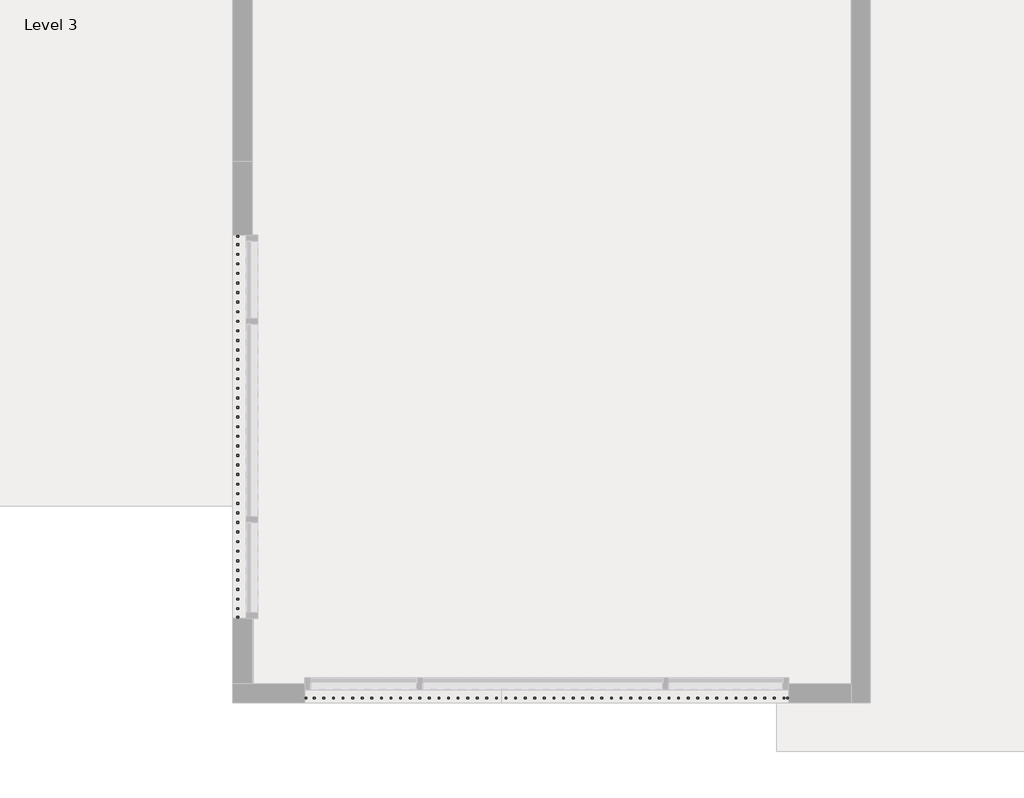
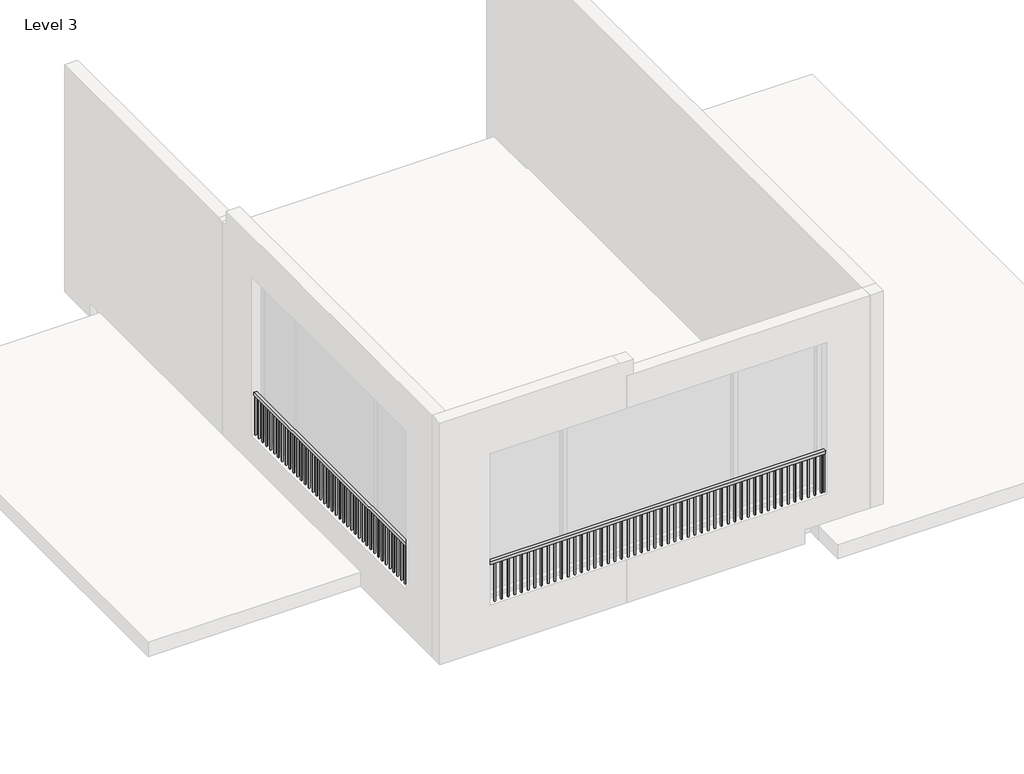
# One storey, part 2 of 2: 2 railings.
"""IFC4 building model written with IfcOpenShell, lengths in millimetres."""

from ifc_helpers import new_model, si_unit, frame, origin, place, context, project, spatial, polyline, outline, extrude, element, save

model = new_model("IFC4")

# Units and contexts
model_context = context("Model", 3, world=origin())
ifc_project = project(units=[si_unit("LENGTHUNIT", "METRE", prefix="MILLI")], contexts=[model_context])

# Site, building, storey
site = spatial("IfcSite", under=ifc_project)
building = spatial("IfcBuilding", under=site)
storey = spatial("IfcBuildingStorey", under=building, Name="Level 3", Elevation=7315.2)

# Railings
placement = place(None, origin())
element("IfcRailing", 1, ObjectType="Handrail - Rectangular", at=placement, inside=storey, context=model_context, shape_type="SweptSolid", body=[
    extrude(outline(polyline([(-11871.2372956, -2267.3372168), (-11871.2372956, -2216.5372168), (-6740.4372956, -2216.5372168), (-6740.4372956, -2267.3372168), (-11871.2372956, -2267.3372168)])), frame((0.0, 0.0, 8636.0), z_axis=(0.0, 0.0, 1.0), x_axis=(1.0, 0.0, 0.0)), (0.0, 0.0, 1.0), 50.8),
    extrude(outline(polyline([(-6800.7622956, -2251.4622168), (-6800.7622956, -2232.4122168), (-6781.7122956, -2232.4122168), (-6781.7122956, -2251.4622168), (-6800.7622956, -2251.4622168)])), frame((0.0, 0.0, 7772.4), z_axis=(0.0, 0.0, 1.0), x_axis=(1.0, 0.0, 0.0)), (0.0, 0.0, 1.0), 863.6),
    extrude(outline(polyline([(-6902.3622956, -2251.4622168), (-6902.3622956, -2232.4122168), (-6883.3122956, -2232.4122168), (-6883.3122956, -2251.4622168), (-6902.3622956, -2251.4622168)])), frame((0.0, 0.0, 7772.4), z_axis=(0.0, 0.0, 1.0), x_axis=(1.0, 0.0, 0.0)), (0.0, 0.0, 1.0), 863.6),
    extrude(outline(polyline([(-7003.9622956, -2251.4622168), (-7003.9622956, -2232.4122168), (-6984.9122956, -2232.4122168), (-6984.9122956, -2251.4622168), (-7003.9622956, -2251.4622168)])), frame((0.0, 0.0, 7772.4), z_axis=(0.0, 0.0, 1.0), x_axis=(1.0, 0.0, 0.0)), (0.0, 0.0, 1.0), 863.6),
    extrude(outline(polyline([(-7105.5622956, -2251.4622168), (-7105.5622956, -2232.4122168), (-7086.5122956, -2232.4122168), (-7086.5122956, -2251.4622168), (-7105.5622956, -2251.4622168)])), frame((0.0, 0.0, 7772.4), z_axis=(0.0, 0.0, 1.0), x_axis=(1.0, 0.0, 0.0)), (0.0, 0.0, 1.0), 863.6),
    extrude(outline(polyline([(-7207.1622956, -2251.4622168), (-7207.1622956, -2232.4122168), (-7188.1122956, -2232.4122168), (-7188.1122956, -2251.4622168), (-7207.1622956, -2251.4622168)])), frame((0.0, 0.0, 7772.4), z_axis=(0.0, 0.0, 1.0), x_axis=(1.0, 0.0, 0.0)), (0.0, 0.0, 1.0), 863.6),
    extrude(outline(polyline([(-7308.7622956, -2251.4622168), (-7308.7622956, -2232.4122168), (-7289.7122956, -2232.4122168), (-7289.7122956, -2251.4622168), (-7308.7622956, -2251.4622168)])), frame((0.0, 0.0, 7772.4), z_axis=(0.0, 0.0, 1.0), x_axis=(1.0, 0.0, 0.0)), (0.0, 0.0, 1.0), 863.6),
    extrude(outline(polyline([(-7410.3622956, -2251.4622168), (-7410.3622956, -2232.4122168), (-7391.3122956, -2232.4122168), (-7391.3122956, -2251.4622168), (-7410.3622956, -2251.4622168)])), frame((0.0, 0.0, 7772.4), z_axis=(0.0, 0.0, 1.0), x_axis=(1.0, 0.0, 0.0)), (0.0, 0.0, 1.0), 863.6),
    extrude(outline(polyline([(-7511.9622956, -2251.4622168), (-7511.9622956, -2232.4122168), (-7492.9122956, -2232.4122168), (-7492.9122956, -2251.4622168), (-7511.9622956, -2251.4622168)])), frame((0.0, 0.0, 7772.4), z_axis=(0.0, 0.0, 1.0), x_axis=(1.0, 0.0, 0.0)), (0.0, 0.0, 1.0), 863.6),
    extrude(outline(polyline([(-7613.5622956, -2251.4622168), (-7613.5622956, -2232.4122168), (-7594.5122956, -2232.4122168), (-7594.5122956, -2251.4622168), (-7613.5622956, -2251.4622168)])), frame((0.0, 0.0, 7772.4), z_axis=(0.0, 0.0, 1.0), x_axis=(1.0, 0.0, 0.0)), (0.0, 0.0, 1.0), 863.6),
    extrude(outline(polyline([(-7715.1622956, -2251.4622168), (-7715.1622956, -2232.4122168), (-7696.1122956, -2232.4122168), (-7696.1122956, -2251.4622168), (-7715.1622956, -2251.4622168)])), frame((0.0, 0.0, 7772.4), z_axis=(0.0, 0.0, 1.0), x_axis=(1.0, 0.0, 0.0)), (0.0, 0.0, 1.0), 863.6),
    extrude(outline(polyline([(-7816.7622956, -2251.4622168), (-7816.7622956, -2232.4122168), (-7797.7122956, -2232.4122168), (-7797.7122956, -2251.4622168), (-7816.7622956, -2251.4622168)])), frame((0.0, 0.0, 7772.4), z_axis=(0.0, 0.0, 1.0), x_axis=(1.0, 0.0, 0.0)), (0.0, 0.0, 1.0), 863.6),
    extrude(outline(polyline([(-7918.3622956, -2251.4622168), (-7918.3622956, -2232.4122168), (-7899.3122956, -2232.4122168), (-7899.3122956, -2251.4622168), (-7918.3622956, -2251.4622168)])), frame((0.0, 0.0, 7772.4), z_axis=(0.0, 0.0, 1.0), x_axis=(1.0, 0.0, 0.0)), (0.0, 0.0, 1.0), 863.6),
    extrude(outline(polyline([(-8019.9622956, -2251.4622168), (-8019.9622956, -2232.4122168), (-8000.9122956, -2232.4122168), (-8000.9122956, -2251.4622168), (-8019.9622956, -2251.4622168)])), frame((0.0, 0.0, 7772.4), z_axis=(0.0, 0.0, 1.0), x_axis=(1.0, 0.0, 0.0)), (0.0, 0.0, 1.0), 863.6),
    extrude(outline(polyline([(-8121.5622956, -2251.4622168), (-8121.5622956, -2232.4122168), (-8102.5122956, -2232.4122168), (-8102.5122956, -2251.4622168), (-8121.5622956, -2251.4622168)])), frame((0.0, 0.0, 7772.4), z_axis=(0.0, 0.0, 1.0), x_axis=(1.0, 0.0, 0.0)), (0.0, 0.0, 1.0), 863.6),
    extrude(outline(polyline([(-8223.1622956, -2251.4622168), (-8223.1622956, -2232.4122168), (-8204.1122956, -2232.4122168), (-8204.1122956, -2251.4622168), (-8223.1622956, -2251.4622168)])), frame((0.0, 0.0, 7772.4), z_axis=(0.0, 0.0, 1.0), x_axis=(1.0, 0.0, 0.0)), (0.0, 0.0, 1.0), 863.6),
    extrude(outline(polyline([(-8324.7622956, -2251.4622168), (-8324.7622956, -2232.4122168), (-8305.7122956, -2232.4122168), (-8305.7122956, -2251.4622168), (-8324.7622956, -2251.4622168)])), frame((0.0, 0.0, 7772.4), z_axis=(0.0, 0.0, 1.0), x_axis=(1.0, 0.0, 0.0)), (0.0, 0.0, 1.0), 863.6),
    extrude(outline(polyline([(-8426.3622956, -2251.4622168), (-8426.3622956, -2232.4122168), (-8407.3122956, -2232.4122168), (-8407.3122956, -2251.4622168), (-8426.3622956, -2251.4622168)])), frame((0.0, 0.0, 7772.4), z_axis=(0.0, 0.0, 1.0), x_axis=(1.0, 0.0, 0.0)), (0.0, 0.0, 1.0), 863.6),
    extrude(outline(polyline([(-8527.9622956, -2251.4622168), (-8527.9622956, -2232.4122168), (-8508.9122956, -2232.4122168), (-8508.9122956, -2251.4622168), (-8527.9622956, -2251.4622168)])), frame((0.0, 0.0, 7772.4), z_axis=(0.0, 0.0, 1.0), x_axis=(1.0, 0.0, 0.0)), (0.0, 0.0, 1.0), 863.6),
    extrude(outline(polyline([(-8629.5622956, -2251.4622168), (-8629.5622956, -2232.4122168), (-8610.5122956, -2232.4122168), (-8610.5122956, -2251.4622168), (-8629.5622956, -2251.4622168)])), frame((0.0, 0.0, 7772.4), z_axis=(0.0, 0.0, 1.0), x_axis=(1.0, 0.0, 0.0)), (0.0, 0.0, 1.0), 863.6),
    extrude(outline(polyline([(-8731.1622956, -2251.4622168), (-8731.1622956, -2232.4122168), (-8712.1122956, -2232.4122168), (-8712.1122956, -2251.4622168), (-8731.1622956, -2251.4622168)])), frame((0.0, 0.0, 7772.4), z_axis=(0.0, 0.0, 1.0), x_axis=(1.0, 0.0, 0.0)), (0.0, 0.0, 1.0), 863.6),
    extrude(outline(polyline([(-8832.7622956, -2251.4622168), (-8832.7622956, -2232.4122168), (-8813.7122956, -2232.4122168), (-8813.7122956, -2251.4622168), (-8832.7622956, -2251.4622168)])), frame((0.0, 0.0, 7772.4), z_axis=(0.0, 0.0, 1.0), x_axis=(1.0, 0.0, 0.0)), (0.0, 0.0, 1.0), 863.6),
    extrude(outline(polyline([(-8934.3622956, -2251.4622168), (-8934.3622956, -2232.4122168), (-8915.3122956, -2232.4122168), (-8915.3122956, -2251.4622168), (-8934.3622956, -2251.4622168)])), frame((0.0, 0.0, 7772.4), z_axis=(0.0, 0.0, 1.0), x_axis=(1.0, 0.0, 0.0)), (0.0, 0.0, 1.0), 863.6),
    extrude(outline(polyline([(-9035.9622956, -2251.4622168), (-9035.9622956, -2232.4122168), (-9016.9122956, -2232.4122168), (-9016.9122956, -2251.4622168), (-9035.9622956, -2251.4622168)])), frame((0.0, 0.0, 7772.4), z_axis=(0.0, 0.0, 1.0), x_axis=(1.0, 0.0, 0.0)), (0.0, 0.0, 1.0), 863.6),
    extrude(outline(polyline([(-9137.5622956, -2251.4622168), (-9137.5622956, -2232.4122168), (-9118.5122956, -2232.4122168), (-9118.5122956, -2251.4622168), (-9137.5622956, -2251.4622168)])), frame((0.0, 0.0, 7772.4), z_axis=(0.0, 0.0, 1.0), x_axis=(1.0, 0.0, 0.0)), (0.0, 0.0, 1.0), 863.6),
    extrude(outline(polyline([(-9239.1622956, -2251.4622168), (-9239.1622956, -2232.4122168), (-9220.1122956, -2232.4122168), (-9220.1122956, -2251.4622168), (-9239.1622956, -2251.4622168)])), frame((0.0, 0.0, 7772.4), z_axis=(0.0, 0.0, 1.0), x_axis=(1.0, 0.0, 0.0)), (0.0, 0.0, 1.0), 863.6),
    extrude(outline(polyline([(-9340.7622956, -2251.4622168), (-9340.7622956, -2232.4122168), (-9321.7122956, -2232.4122168), (-9321.7122956, -2251.4622168), (-9340.7622956, -2251.4622168)])), frame((0.0, 0.0, 7772.4), z_axis=(0.0, 0.0, 1.0), x_axis=(1.0, 0.0, 0.0)), (0.0, 0.0, 1.0), 863.6),
    extrude(outline(polyline([(-9442.3622956, -2251.4622168), (-9442.3622956, -2232.4122168), (-9423.3122956, -2232.4122168), (-9423.3122956, -2251.4622168), (-9442.3622956, -2251.4622168)])), frame((0.0, 0.0, 7772.4), z_axis=(0.0, 0.0, 1.0), x_axis=(1.0, 0.0, 0.0)), (0.0, 0.0, 1.0), 863.6),
    extrude(outline(polyline([(-9543.9622956, -2251.4622168), (-9543.9622956, -2232.4122168), (-9524.9122956, -2232.4122168), (-9524.9122956, -2251.4622168), (-9543.9622956, -2251.4622168)])), frame((0.0, 0.0, 7772.4), z_axis=(0.0, 0.0, 1.0), x_axis=(1.0, 0.0, 0.0)), (0.0, 0.0, 1.0), 863.6),
    extrude(outline(polyline([(-9645.5622956, -2251.4622168), (-9645.5622956, -2232.4122168), (-9626.5122956, -2232.4122168), (-9626.5122956, -2251.4622168), (-9645.5622956, -2251.4622168)])), frame((0.0, 0.0, 7772.4), z_axis=(0.0, 0.0, 1.0), x_axis=(1.0, 0.0, 0.0)), (0.0, 0.0, 1.0), 863.6),
    extrude(outline(polyline([(-9747.1622956, -2251.4622168), (-9747.1622956, -2232.4122168), (-9728.1122956, -2232.4122168), (-9728.1122956, -2251.4622168), (-9747.1622956, -2251.4622168)])), frame((0.0, 0.0, 7772.4), z_axis=(0.0, 0.0, 1.0), x_axis=(1.0, 0.0, 0.0)), (0.0, 0.0, 1.0), 863.6),
    extrude(outline(polyline([(-9848.7622956, -2251.4622168), (-9848.7622956, -2232.4122168), (-9829.7122956, -2232.4122168), (-9829.7122956, -2251.4622168), (-9848.7622956, -2251.4622168)])), frame((0.0, 0.0, 7772.4), z_axis=(0.0, 0.0, 1.0), x_axis=(1.0, 0.0, 0.0)), (0.0, 0.0, 1.0), 863.6),
    extrude(outline(polyline([(-9950.3622956, -2251.4622168), (-9950.3622956, -2232.4122168), (-9931.3122956, -2232.4122168), (-9931.3122956, -2251.4622168), (-9950.3622956, -2251.4622168)])), frame((0.0, 0.0, 7772.4), z_axis=(0.0, 0.0, 1.0), x_axis=(1.0, 0.0, 0.0)), (0.0, 0.0, 1.0), 863.6),
    extrude(outline(polyline([(-10051.9622956, -2251.4622168), (-10051.9622956, -2232.4122168), (-10032.9122956, -2232.4122168), (-10032.9122956, -2251.4622168), (-10051.9622956, -2251.4622168)])), frame((0.0, 0.0, 7772.4), z_axis=(0.0, 0.0, 1.0), x_axis=(1.0, 0.0, 0.0)), (0.0, 0.0, 1.0), 863.6),
    extrude(outline(polyline([(-10153.5622956, -2251.4622168), (-10153.5622956, -2232.4122168), (-10134.5122956, -2232.4122168), (-10134.5122956, -2251.4622168), (-10153.5622956, -2251.4622168)])), frame((0.0, 0.0, 7772.4), z_axis=(0.0, 0.0, 1.0), x_axis=(1.0, 0.0, 0.0)), (0.0, 0.0, 1.0), 863.6),
    extrude(outline(polyline([(-10255.1622956, -2251.4622168), (-10255.1622956, -2232.4122168), (-10236.1122956, -2232.4122168), (-10236.1122956, -2251.4622168), (-10255.1622956, -2251.4622168)])), frame((0.0, 0.0, 7772.4), z_axis=(0.0, 0.0, 1.0), x_axis=(1.0, 0.0, 0.0)), (0.0, 0.0, 1.0), 863.6),
    extrude(outline(polyline([(-10356.7622956, -2251.4622168), (-10356.7622956, -2232.4122168), (-10337.7122956, -2232.4122168), (-10337.7122956, -2251.4622168), (-10356.7622956, -2251.4622168)])), frame((0.0, 0.0, 7772.4), z_axis=(0.0, 0.0, 1.0), x_axis=(1.0, 0.0, 0.0)), (0.0, 0.0, 1.0), 863.6),
    extrude(outline(polyline([(-10458.3622956, -2251.4622168), (-10458.3622956, -2232.4122168), (-10439.3122956, -2232.4122168), (-10439.3122956, -2251.4622168), (-10458.3622956, -2251.4622168)])), frame((0.0, 0.0, 7772.4), z_axis=(0.0, 0.0, 1.0), x_axis=(1.0, 0.0, 0.0)), (0.0, 0.0, 1.0), 863.6),
    extrude(outline(polyline([(-10559.9622956, -2251.4622168), (-10559.9622956, -2232.4122168), (-10540.9122956, -2232.4122168), (-10540.9122956, -2251.4622168), (-10559.9622956, -2251.4622168)])), frame((0.0, 0.0, 7772.4), z_axis=(0.0, 0.0, 1.0), x_axis=(1.0, 0.0, 0.0)), (0.0, 0.0, 1.0), 863.6),
    extrude(outline(polyline([(-10661.5622956, -2251.4622168), (-10661.5622956, -2232.4122168), (-10642.5122956, -2232.4122168), (-10642.5122956, -2251.4622168), (-10661.5622956, -2251.4622168)])), frame((0.0, 0.0, 7772.4), z_axis=(0.0, 0.0, 1.0), x_axis=(1.0, 0.0, 0.0)), (0.0, 0.0, 1.0), 863.6),
    extrude(outline(polyline([(-10763.1622956, -2251.4622168), (-10763.1622956, -2232.4122168), (-10744.1122956, -2232.4122168), (-10744.1122956, -2251.4622168), (-10763.1622956, -2251.4622168)])), frame((0.0, 0.0, 7772.4), z_axis=(0.0, 0.0, 1.0), x_axis=(1.0, 0.0, 0.0)), (0.0, 0.0, 1.0), 863.6),
    extrude(outline(polyline([(-10864.7622956, -2251.4622168), (-10864.7622956, -2232.4122168), (-10845.7122956, -2232.4122168), (-10845.7122956, -2251.4622168), (-10864.7622956, -2251.4622168)])), frame((0.0, 0.0, 7772.4), z_axis=(0.0, 0.0, 1.0), x_axis=(1.0, 0.0, 0.0)), (0.0, 0.0, 1.0), 863.6),
    extrude(outline(polyline([(-10966.3622956, -2251.4622168), (-10966.3622956, -2232.4122168), (-10947.3122956, -2232.4122168), (-10947.3122956, -2251.4622168), (-10966.3622956, -2251.4622168)])), frame((0.0, 0.0, 7772.4), z_axis=(0.0, 0.0, 1.0), x_axis=(1.0, 0.0, 0.0)), (0.0, 0.0, 1.0), 863.6),
    extrude(outline(polyline([(-11067.9622956, -2251.4622168), (-11067.9622956, -2232.4122168), (-11048.9122956, -2232.4122168), (-11048.9122956, -2251.4622168), (-11067.9622956, -2251.4622168)])), frame((0.0, 0.0, 7772.4), z_axis=(0.0, 0.0, 1.0), x_axis=(1.0, 0.0, 0.0)), (0.0, 0.0, 1.0), 863.6),
    extrude(outline(polyline([(-11169.5622956, -2251.4622168), (-11169.5622956, -2232.4122168), (-11150.5122956, -2232.4122168), (-11150.5122956, -2251.4622168), (-11169.5622956, -2251.4622168)])), frame((0.0, 0.0, 7772.4), z_axis=(0.0, 0.0, 1.0), x_axis=(1.0, 0.0, 0.0)), (0.0, 0.0, 1.0), 863.6),
    extrude(outline(polyline([(-11271.1622956, -2251.4622168), (-11271.1622956, -2232.4122168), (-11252.1122956, -2232.4122168), (-11252.1122956, -2251.4622168), (-11271.1622956, -2251.4622168)])), frame((0.0, 0.0, 7772.4), z_axis=(0.0, 0.0, 1.0), x_axis=(1.0, 0.0, 0.0)), (0.0, 0.0, 1.0), 863.6),
    extrude(outline(polyline([(-11372.7622956, -2251.4622168), (-11372.7622956, -2232.4122168), (-11353.7122956, -2232.4122168), (-11353.7122956, -2251.4622168), (-11372.7622956, -2251.4622168)])), frame((0.0, 0.0, 7772.4), z_axis=(0.0, 0.0, 1.0), x_axis=(1.0, 0.0, 0.0)), (0.0, 0.0, 1.0), 863.6),
    extrude(outline(polyline([(-11474.3622956, -2251.4622168), (-11474.3622956, -2232.4122168), (-11455.3122956, -2232.4122168), (-11455.3122956, -2251.4622168), (-11474.3622956, -2251.4622168)])), frame((0.0, 0.0, 7772.4), z_axis=(0.0, 0.0, 1.0), x_axis=(1.0, 0.0, 0.0)), (0.0, 0.0, 1.0), 863.6),
    extrude(outline(polyline([(-11575.9622956, -2251.4622168), (-11575.9622956, -2232.4122168), (-11556.9122956, -2232.4122168), (-11556.9122956, -2251.4622168), (-11575.9622956, -2251.4622168)])), frame((0.0, 0.0, 7772.4), z_axis=(0.0, 0.0, 1.0), x_axis=(1.0, 0.0, 0.0)), (0.0, 0.0, 1.0), 863.6),
    extrude(outline(polyline([(-11677.5622956, -2251.4622168), (-11677.5622956, -2232.4122168), (-11658.5122956, -2232.4122168), (-11658.5122956, -2251.4622168), (-11677.5622956, -2251.4622168)])), frame((0.0, 0.0, 7772.4), z_axis=(0.0, 0.0, 1.0), x_axis=(1.0, 0.0, 0.0)), (0.0, 0.0, 1.0), 863.6),
    extrude(outline(polyline([(-11779.1622956, -2251.4622168), (-11779.1622956, -2232.4122168), (-11760.1122956, -2232.4122168), (-11760.1122956, -2251.4622168), (-11779.1622956, -2251.4622168)])), frame((0.0, 0.0, 7772.4), z_axis=(0.0, 0.0, 1.0), x_axis=(1.0, 0.0, 0.0)), (0.0, 0.0, 1.0), 863.6),
    extrude(outline(polyline([(-6759.4872956, -2251.4622168), (-6759.4872956, -2232.4122168), (-6740.4372956, -2232.4122168), (-6740.4372956, -2251.4622168), (-6759.4872956, -2251.4622168)])), frame((0.0, 0.0, 7772.4), z_axis=(0.0, 0.0, 1.0), x_axis=(1.0, 0.0, 0.0)), (0.0, 0.0, 1.0), 863.6),
    extrude(outline(polyline([(-11871.2372956, -2251.4622168), (-11871.2372956, -2232.4122168), (-11852.1872956, -2232.4122168), (-11852.1872956, -2251.4622168), (-11871.2372956, -2251.4622168)])), frame((0.0, 0.0, 7772.4), z_axis=(0.0, 0.0, 1.0), x_axis=(1.0, 0.0, 0.0)), (0.0, 0.0, 1.0), 863.6),
])
element("IfcRailing", 2, ObjectType="Handrail - Rectangular", at=placement, inside=storey, context=model_context, shape_type="SweptSolid", body=[
    extrude(outline(polyline([(-12607.8372956, 2667.561619), (-12557.0372956, 2667.561619), (-12557.0372956, -1396.438381), (-12607.8372956, -1396.438381), (-12607.8372956, 2667.561619)])), frame((0.0, 0.0, 8636.0), z_axis=(0.0, 0.0, 1.0), x_axis=(1.0, 0.0, 0.0)), (0.0, 0.0, 1.0), 50.8),
    extrude(outline(polyline([(-12591.9622956, -1285.313381), (-12572.9122956, -1285.313381), (-12572.9122956, -1304.363381), (-12591.9622956, -1304.363381), (-12591.9622956, -1285.313381)])), frame((0.0, 0.0, 7772.4), z_axis=(0.0, 0.0, 1.0), x_axis=(1.0, 0.0, 0.0)), (0.0, 0.0, 1.0), 863.6),
    extrude(outline(polyline([(-12591.9622956, -1183.713381), (-12572.9122956, -1183.713381), (-12572.9122956, -1202.763381), (-12591.9622956, -1202.763381), (-12591.9622956, -1183.713381)])), frame((0.0, 0.0, 7772.4), z_axis=(0.0, 0.0, 1.0), x_axis=(1.0, 0.0, 0.0)), (0.0, 0.0, 1.0), 863.6),
    extrude(outline(polyline([(-12591.9622956, -1082.113381), (-12572.9122956, -1082.113381), (-12572.9122956, -1101.163381), (-12591.9622956, -1101.163381), (-12591.9622956, -1082.113381)])), frame((0.0, 0.0, 7772.4), z_axis=(0.0, 0.0, 1.0), x_axis=(1.0, 0.0, 0.0)), (0.0, 0.0, 1.0), 863.6),
    extrude(outline(polyline([(-12591.9622956, -980.513381), (-12572.9122956, -980.513381), (-12572.9122956, -999.563381), (-12591.9622956, -999.563381), (-12591.9622956, -980.513381)])), frame((0.0, 0.0, 7772.4), z_axis=(0.0, 0.0, 1.0), x_axis=(1.0, 0.0, 0.0)), (0.0, 0.0, 1.0), 863.6),
    extrude(outline(polyline([(-12591.9622956, -878.913381), (-12572.9122956, -878.913381), (-12572.9122956, -897.963381), (-12591.9622956, -897.963381), (-12591.9622956, -878.913381)])), frame((0.0, 0.0, 7772.4), z_axis=(0.0, 0.0, 1.0), x_axis=(1.0, 0.0, 0.0)), (0.0, 0.0, 1.0), 863.6),
    extrude(outline(polyline([(-12591.9622956, -777.313381), (-12572.9122956, -777.313381), (-12572.9122956, -796.363381), (-12591.9622956, -796.363381), (-12591.9622956, -777.313381)])), frame((0.0, 0.0, 7772.4), z_axis=(0.0, 0.0, 1.0), x_axis=(1.0, 0.0, 0.0)), (0.0, 0.0, 1.0), 863.6),
    extrude(outline(polyline([(-12591.9622956, -675.713381), (-12572.9122956, -675.713381), (-12572.9122956, -694.763381), (-12591.9622956, -694.763381), (-12591.9622956, -675.713381)])), frame((0.0, 0.0, 7772.4), z_axis=(0.0, 0.0, 1.0), x_axis=(1.0, 0.0, 0.0)), (0.0, 0.0, 1.0), 863.6),
    extrude(outline(polyline([(-12591.9622956, -574.113381), (-12572.9122956, -574.113381), (-12572.9122956, -593.163381), (-12591.9622956, -593.163381), (-12591.9622956, -574.113381)])), frame((0.0, 0.0, 7772.4), z_axis=(0.0, 0.0, 1.0), x_axis=(1.0, 0.0, 0.0)), (0.0, 0.0, 1.0), 863.6),
    extrude(outline(polyline([(-12591.9622956, -472.513381), (-12572.9122956, -472.513381), (-12572.9122956, -491.563381), (-12591.9622956, -491.563381), (-12591.9622956, -472.513381)])), frame((0.0, 0.0, 7772.4), z_axis=(0.0, 0.0, 1.0), x_axis=(1.0, 0.0, 0.0)), (0.0, 0.0, 1.0), 863.6),
    extrude(outline(polyline([(-12591.9622956, -370.913381), (-12572.9122956, -370.913381), (-12572.9122956, -389.963381), (-12591.9622956, -389.963381), (-12591.9622956, -370.913381)])), frame((0.0, 0.0, 7772.4), z_axis=(0.0, 0.0, 1.0), x_axis=(1.0, 0.0, 0.0)), (0.0, 0.0, 1.0), 863.6),
    extrude(outline(polyline([(-12591.9622956, -269.313381), (-12572.9122956, -269.313381), (-12572.9122956, -288.363381), (-12591.9622956, -288.363381), (-12591.9622956, -269.313381)])), frame((0.0, 0.0, 7772.4), z_axis=(0.0, 0.0, 1.0), x_axis=(1.0, 0.0, 0.0)), (0.0, 0.0, 1.0), 863.6),
    extrude(outline(polyline([(-12591.9622956, -167.713381), (-12572.9122956, -167.713381), (-12572.9122956, -186.763381), (-12591.9622956, -186.763381), (-12591.9622956, -167.713381)])), frame((0.0, 0.0, 7772.4), z_axis=(0.0, 0.0, 1.0), x_axis=(1.0, 0.0, 0.0)), (0.0, 0.0, 1.0), 863.6),
    extrude(outline(polyline([(-12591.9622956, -66.113381), (-12572.9122956, -66.113381), (-12572.9122956, -85.163381), (-12591.9622956, -85.163381), (-12591.9622956, -66.113381)])), frame((0.0, 0.0, 7772.4), z_axis=(0.0, 0.0, 1.0), x_axis=(1.0, 0.0, 0.0)), (0.0, 0.0, 1.0), 863.6),
    extrude(outline(polyline([(-12591.9622956, 35.486619), (-12572.9122956, 35.486619), (-12572.9122956, 16.436619), (-12591.9622956, 16.436619), (-12591.9622956, 35.486619)])), frame((0.0, 0.0, 7772.4), z_axis=(0.0, 0.0, 1.0), x_axis=(1.0, 0.0, 0.0)), (0.0, 0.0, 1.0), 863.6),
    extrude(outline(polyline([(-12591.9622956, 137.086619), (-12572.9122956, 137.086619), (-12572.9122956, 118.036619), (-12591.9622956, 118.036619), (-12591.9622956, 137.086619)])), frame((0.0, 0.0, 7772.4), z_axis=(0.0, 0.0, 1.0), x_axis=(1.0, 0.0, 0.0)), (0.0, 0.0, 1.0), 863.6),
    extrude(outline(polyline([(-12591.9622956, 238.686619), (-12572.9122956, 238.686619), (-12572.9122956, 219.636619), (-12591.9622956, 219.636619), (-12591.9622956, 238.686619)])), frame((0.0, 0.0, 7772.4), z_axis=(0.0, 0.0, 1.0), x_axis=(1.0, 0.0, 0.0)), (0.0, 0.0, 1.0), 863.6),
    extrude(outline(polyline([(-12591.9622956, 340.286619), (-12572.9122956, 340.286619), (-12572.9122956, 321.236619), (-12591.9622956, 321.236619), (-12591.9622956, 340.286619)])), frame((0.0, 0.0, 7772.4), z_axis=(0.0, 0.0, 1.0), x_axis=(1.0, 0.0, 0.0)), (0.0, 0.0, 1.0), 863.6),
    extrude(outline(polyline([(-12591.9622956, 441.886619), (-12572.9122956, 441.886619), (-12572.9122956, 422.836619), (-12591.9622956, 422.836619), (-12591.9622956, 441.886619)])), frame((0.0, 0.0, 7772.4), z_axis=(0.0, 0.0, 1.0), x_axis=(1.0, 0.0, 0.0)), (0.0, 0.0, 1.0), 863.6),
    extrude(outline(polyline([(-12591.9622956, 543.486619), (-12572.9122956, 543.486619), (-12572.9122956, 524.436619), (-12591.9622956, 524.436619), (-12591.9622956, 543.486619)])), frame((0.0, 0.0, 7772.4), z_axis=(0.0, 0.0, 1.0), x_axis=(1.0, 0.0, 0.0)), (0.0, 0.0, 1.0), 863.6),
    extrude(outline(polyline([(-12591.9622956, 645.086619), (-12572.9122956, 645.086619), (-12572.9122956, 626.036619), (-12591.9622956, 626.036619), (-12591.9622956, 645.086619)])), frame((0.0, 0.0, 7772.4), z_axis=(0.0, 0.0, 1.0), x_axis=(1.0, 0.0, 0.0)), (0.0, 0.0, 1.0), 863.6),
    extrude(outline(polyline([(-12591.9622956, 746.686619), (-12572.9122956, 746.686619), (-12572.9122956, 727.636619), (-12591.9622956, 727.636619), (-12591.9622956, 746.686619)])), frame((0.0, 0.0, 7772.4), z_axis=(0.0, 0.0, 1.0), x_axis=(1.0, 0.0, 0.0)), (0.0, 0.0, 1.0), 863.6),
    extrude(outline(polyline([(-12591.9622956, 848.286619), (-12572.9122956, 848.286619), (-12572.9122956, 829.236619), (-12591.9622956, 829.236619), (-12591.9622956, 848.286619)])), frame((0.0, 0.0, 7772.4), z_axis=(0.0, 0.0, 1.0), x_axis=(1.0, 0.0, 0.0)), (0.0, 0.0, 1.0), 863.6),
    extrude(outline(polyline([(-12591.9622956, 949.886619), (-12572.9122956, 949.886619), (-12572.9122956, 930.836619), (-12591.9622956, 930.836619), (-12591.9622956, 949.886619)])), frame((0.0, 0.0, 7772.4), z_axis=(0.0, 0.0, 1.0), x_axis=(1.0, 0.0, 0.0)), (0.0, 0.0, 1.0), 863.6),
    extrude(outline(polyline([(-12591.9622956, 1051.486619), (-12572.9122956, 1051.486619), (-12572.9122956, 1032.436619), (-12591.9622956, 1032.436619), (-12591.9622956, 1051.486619)])), frame((0.0, 0.0, 7772.4), z_axis=(0.0, 0.0, 1.0), x_axis=(1.0, 0.0, 0.0)), (0.0, 0.0, 1.0), 863.6),
    extrude(outline(polyline([(-12591.9622956, 1153.086619), (-12572.9122956, 1153.086619), (-12572.9122956, 1134.036619), (-12591.9622956, 1134.036619), (-12591.9622956, 1153.086619)])), frame((0.0, 0.0, 7772.4), z_axis=(0.0, 0.0, 1.0), x_axis=(1.0, 0.0, 0.0)), (0.0, 0.0, 1.0), 863.6),
    extrude(outline(polyline([(-12591.9622956, 1254.686619), (-12572.9122956, 1254.686619), (-12572.9122956, 1235.636619), (-12591.9622956, 1235.636619), (-12591.9622956, 1254.686619)])), frame((0.0, 0.0, 7772.4), z_axis=(0.0, 0.0, 1.0), x_axis=(1.0, 0.0, 0.0)), (0.0, 0.0, 1.0), 863.6),
    extrude(outline(polyline([(-12591.9622956, 1356.286619), (-12572.9122956, 1356.286619), (-12572.9122956, 1337.236619), (-12591.9622956, 1337.236619), (-12591.9622956, 1356.286619)])), frame((0.0, 0.0, 7772.4), z_axis=(0.0, 0.0, 1.0), x_axis=(1.0, 0.0, 0.0)), (0.0, 0.0, 1.0), 863.6),
    extrude(outline(polyline([(-12591.9622956, 1457.886619), (-12572.9122956, 1457.886619), (-12572.9122956, 1438.836619), (-12591.9622956, 1438.836619), (-12591.9622956, 1457.886619)])), frame((0.0, 0.0, 7772.4), z_axis=(0.0, 0.0, 1.0), x_axis=(1.0, 0.0, 0.0)), (0.0, 0.0, 1.0), 863.6),
    extrude(outline(polyline([(-12591.9622956, 1559.486619), (-12572.9122956, 1559.486619), (-12572.9122956, 1540.436619), (-12591.9622956, 1540.436619), (-12591.9622956, 1559.486619)])), frame((0.0, 0.0, 7772.4), z_axis=(0.0, 0.0, 1.0), x_axis=(1.0, 0.0, 0.0)), (0.0, 0.0, 1.0), 863.6),
    extrude(outline(polyline([(-12591.9622956, 1661.086619), (-12572.9122956, 1661.086619), (-12572.9122956, 1642.036619), (-12591.9622956, 1642.036619), (-12591.9622956, 1661.086619)])), frame((0.0, 0.0, 7772.4), z_axis=(0.0, 0.0, 1.0), x_axis=(1.0, 0.0, 0.0)), (0.0, 0.0, 1.0), 863.6),
    extrude(outline(polyline([(-12591.9622956, 1762.686619), (-12572.9122956, 1762.686619), (-12572.9122956, 1743.636619), (-12591.9622956, 1743.636619), (-12591.9622956, 1762.686619)])), frame((0.0, 0.0, 7772.4), z_axis=(0.0, 0.0, 1.0), x_axis=(1.0, 0.0, 0.0)), (0.0, 0.0, 1.0), 863.6),
    extrude(outline(polyline([(-12591.9622956, 1864.286619), (-12572.9122956, 1864.286619), (-12572.9122956, 1845.236619), (-12591.9622956, 1845.236619), (-12591.9622956, 1864.286619)])), frame((0.0, 0.0, 7772.4), z_axis=(0.0, 0.0, 1.0), x_axis=(1.0, 0.0, 0.0)), (0.0, 0.0, 1.0), 863.6),
    extrude(outline(polyline([(-12591.9622956, 1965.886619), (-12572.9122956, 1965.886619), (-12572.9122956, 1946.836619), (-12591.9622956, 1946.836619), (-12591.9622956, 1965.886619)])), frame((0.0, 0.0, 7772.4), z_axis=(0.0, 0.0, 1.0), x_axis=(1.0, 0.0, 0.0)), (0.0, 0.0, 1.0), 863.6),
    extrude(outline(polyline([(-12591.9622956, 2067.486619), (-12572.9122956, 2067.486619), (-12572.9122956, 2048.436619), (-12591.9622956, 2048.436619), (-12591.9622956, 2067.486619)])), frame((0.0, 0.0, 7772.4), z_axis=(0.0, 0.0, 1.0), x_axis=(1.0, 0.0, 0.0)), (0.0, 0.0, 1.0), 863.6),
    extrude(outline(polyline([(-12591.9622956, 2169.086619), (-12572.9122956, 2169.086619), (-12572.9122956, 2150.036619), (-12591.9622956, 2150.036619), (-12591.9622956, 2169.086619)])), frame((0.0, 0.0, 7772.4), z_axis=(0.0, 0.0, 1.0), x_axis=(1.0, 0.0, 0.0)), (0.0, 0.0, 1.0), 863.6),
    extrude(outline(polyline([(-12591.9622956, 2270.686619), (-12572.9122956, 2270.686619), (-12572.9122956, 2251.636619), (-12591.9622956, 2251.636619), (-12591.9622956, 2270.686619)])), frame((0.0, 0.0, 7772.4), z_axis=(0.0, 0.0, 1.0), x_axis=(1.0, 0.0, 0.0)), (0.0, 0.0, 1.0), 863.6),
    extrude(outline(polyline([(-12591.9622956, 2372.286619), (-12572.9122956, 2372.286619), (-12572.9122956, 2353.236619), (-12591.9622956, 2353.236619), (-12591.9622956, 2372.286619)])), frame((0.0, 0.0, 7772.4), z_axis=(0.0, 0.0, 1.0), x_axis=(1.0, 0.0, 0.0)), (0.0, 0.0, 1.0), 863.6),
    extrude(outline(polyline([(-12591.9622956, 2473.886619), (-12572.9122956, 2473.886619), (-12572.9122956, 2454.836619), (-12591.9622956, 2454.836619), (-12591.9622956, 2473.886619)])), frame((0.0, 0.0, 7772.4), z_axis=(0.0, 0.0, 1.0), x_axis=(1.0, 0.0, 0.0)), (0.0, 0.0, 1.0), 863.6),
    extrude(outline(polyline([(-12591.9622956, 2575.486619), (-12572.9122956, 2575.486619), (-12572.9122956, 2556.436619), (-12591.9622956, 2556.436619), (-12591.9622956, 2575.486619)])), frame((0.0, 0.0, 7772.4), z_axis=(0.0, 0.0, 1.0), x_axis=(1.0, 0.0, 0.0)), (0.0, 0.0, 1.0), 863.6),
    extrude(outline(polyline([(-12591.9622956, -1377.388381), (-12572.9122956, -1377.388381), (-12572.9122956, -1396.438381), (-12591.9622956, -1396.438381), (-12591.9622956, -1377.388381)])), frame((0.0, 0.0, 7772.4), z_axis=(0.0, 0.0, 1.0), x_axis=(1.0, 0.0, 0.0)), (0.0, 0.0, 1.0), 863.6),
    extrude(outline(polyline([(-12591.9622956, 2667.561619), (-12572.9122956, 2667.561619), (-12572.9122956, 2648.511619), (-12591.9622956, 2648.511619), (-12591.9622956, 2667.561619)])), frame((0.0, 0.0, 7772.4), z_axis=(0.0, 0.0, 1.0), x_axis=(1.0, 0.0, 0.0)), (0.0, 0.0, 1.0), 863.6),
])

save(model, "model.ifc")

# Revit data of these elements
# Type "Handrail - Rectangular"
#   Assembly Code = "C2010400"
#   built-in parameter 1008612 = 0.0416667 (stored number, unit not read)
#   built-in parameter 1008611 = 0.0416667 (stored number, unit not read)
#   built-in parameter 1008609 = 0.333333 (stored number, unit not read)
#   built-in parameter 1008604 = 0.166667 (stored number, unit not read)
#   built-in parameter 1008603 = 0.166667 (stored number, unit not read)
#   Railing Height = 3' - 0"
#   built-in parameter 1008630 = 2
#   built-in parameter 1008610 = 2
#   built-in parameter 1008618 = Baluster - Square : 3/4"
# Elements 1, 2 (IfcRailing, "Handrail - Rectangular")
#   built-in parameter 1008621 = 1.5 (stored number, unit not read)
#   Phase Created = New Construction
